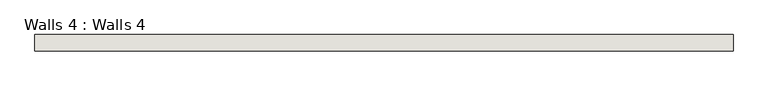
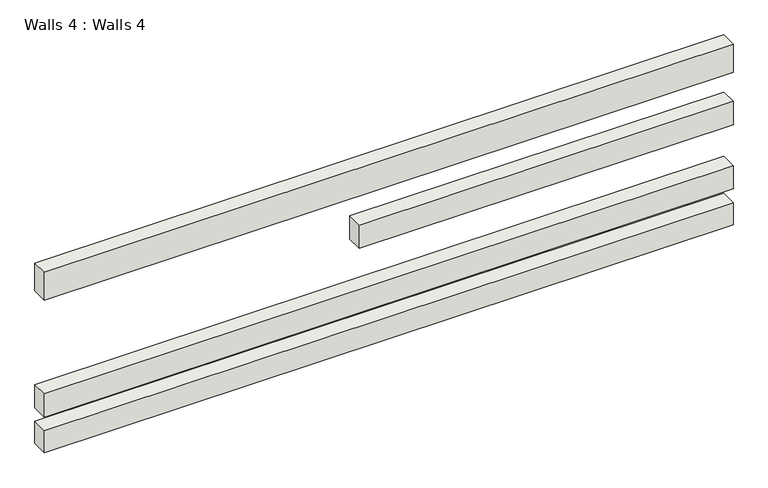
"""IFC4 building model written with IfcOpenShell, lengths in millimetres: wall geometry, Walls 4 : Walls 4."""

from ifc_helpers import new_model, si_unit, frame, origin, place, context, project, spatial, polyline, outline, extrude, source, transform, mapped, element, save


def walls_4_walls_4_47acbb33(model_context):
    return source(origin(), model_context, "Body", "SweptSolid", [
        extrude(outline(polyline([(-6704.9165692, -432.5886674), (-12038.9165692, -432.5886674), (-12038.9165692, -306.6724828), (-6704.9165692, -306.6724828), (-6704.9165692, -432.5886674)])), frame((0.0, 0.0, 1439.3828444), z_axis=(0.0, 0.0, 1.0), x_axis=(1.0, 0.0, 0.0)), (0.0, 0.0, 1.0), 228.6),
        extrude(outline(polyline([(-6704.9165692, -432.5886674), (-9599.867741, -432.5886674), (-9599.867741, -306.6724828), (-6704.9165692, -306.6724828), (-6704.9165692, -432.5886674)])), frame((0.0, 0.0, 1010.2258788), z_axis=(0.0, 0.0, 1.0), x_axis=(1.0, 0.0, 0.0)), (0.0, 0.0, 1.0), 189.8392414),
        extrude(outline(polyline([(-6704.9165692, -432.5886674), (-12038.9165692, -432.5886674), (-12038.9165692, -306.6724828), (-6704.9165692, -306.6724828), (-6704.9165692, -432.5886674)])), frame((0.0, 0.0, 482.9611246), z_axis=(0.0, 0.0, 1.0), x_axis=(1.0, 0.0, 0.0)), (0.0, 0.0, 1.0), 189.8392414),
        extrude(outline(polyline([(-6704.9165692, -432.5886674), (-12038.9165692, -432.5886674), (-12038.9165692, -306.6724828), (-6704.9165692, -306.6724828), (-6704.9165692, -432.5886674)])), frame((0.0, 0.0, 191.1225694), z_axis=(0.0, 0.0, 1.0), x_axis=(1.0, 0.0, 0.0)), (0.0, 0.0, 1.0), 179.9192054),
    ])


if __name__ == "__main__":
    model = new_model("IFC4")
    model_context = context("Model", 3, world=origin())
    ifc_project = project(units=[si_unit("LENGTHUNIT", "METRE", prefix="MILLI")], contexts=[model_context])
    site = spatial("IfcSite", under=ifc_project)
    building = spatial("IfcBuilding", under=site)
    placement = place(None, origin())
    walls_4_walls_4_shape = walls_4_walls_4_47acbb33(model_context)
    element("IfcWall", 1, ObjectType="Walls 4 : Walls 4", at=placement, inside=building, context=model_context, shape_type="MappedRepresentation", body=[
        mapped(walls_4_walls_4_shape, transform((0.0, 0.0, 0.0), x_axis=(1.0, 0.0, 0.0), y_axis=(0.0, 1.0, 0.0), z_axis=(0.0, 0.0, 1.0))),
    ])
    save(model, "model.ifc")

# Revit data of these elements
# Element 1 (IfcWall, "Walls 4 : Walls 4")
#   Materials on its faces: "Default Wall"
# Materials
#   "Default Wall": colour RGB 128 128 128, transparency 0
